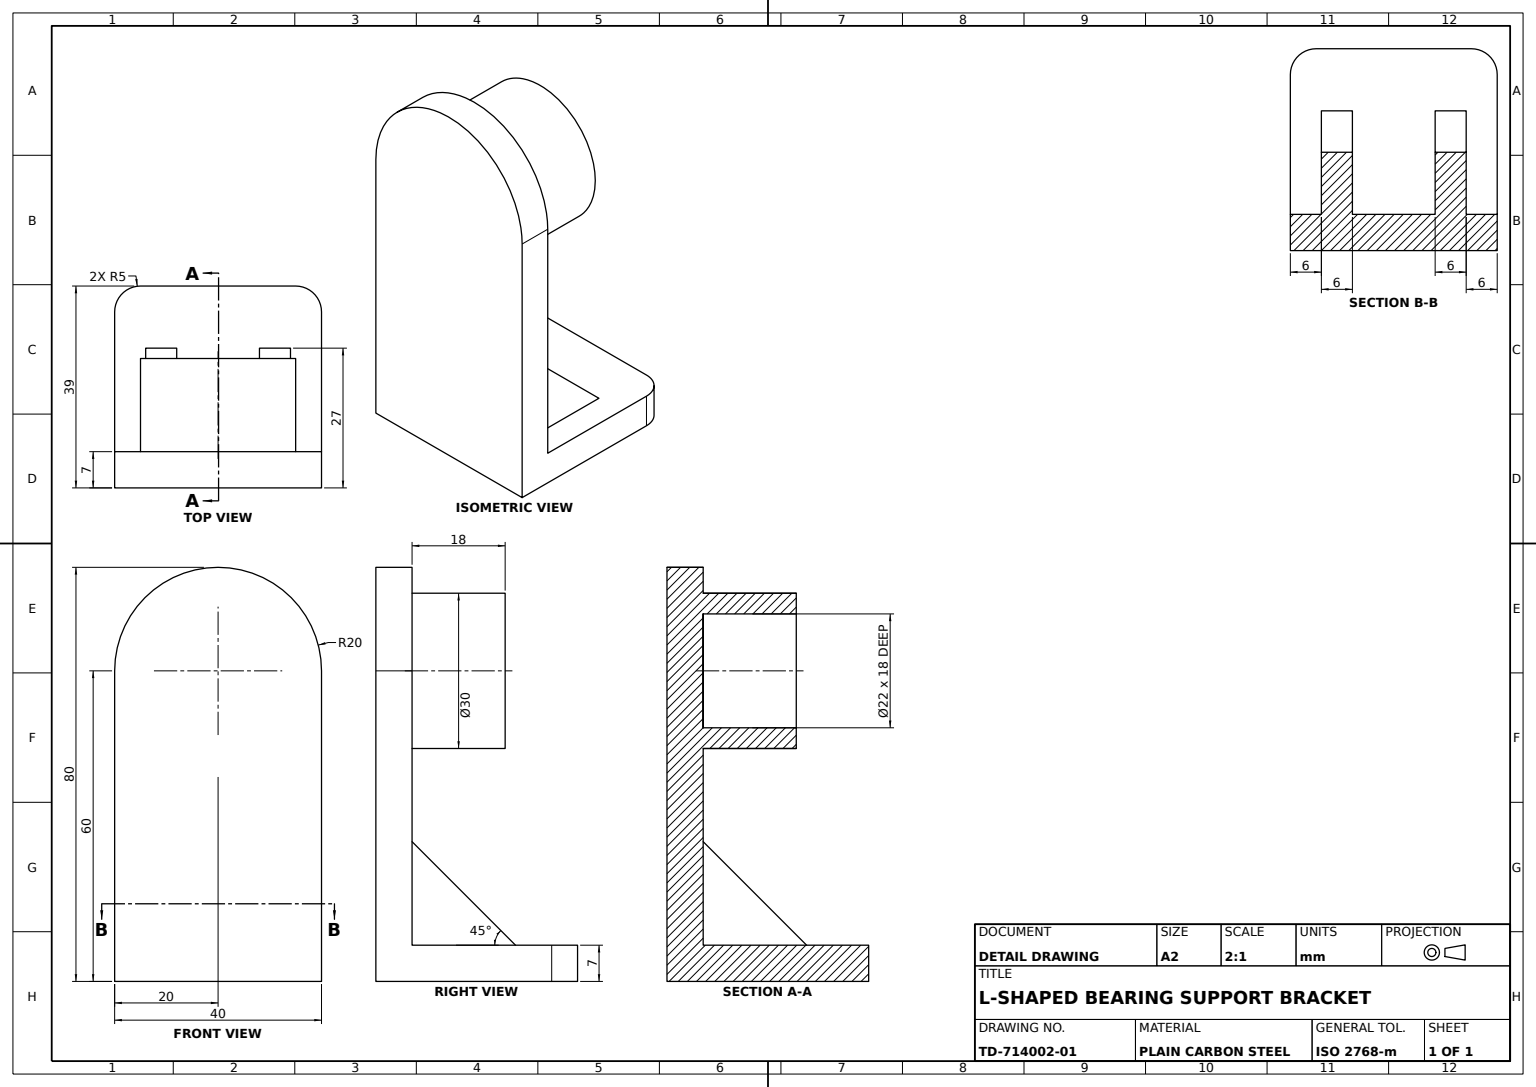
from build123d import *

# Parameters (mm, degrees)
L_BRACKET_BASE_DEPTH      = 40
CORNER_BLOCK_DEPTH        = 7
UPRIGHT_ROUNDED_TOP_DEPTH = 7
HUB_SKETCH_30_R           = 15
HUB_30_DEPTH              = 18
BORE_SKETCH_22_R          = 11
BORE_22_DEPTH             = 18
RIB_1_DEPTH               = 12
RIB_2_DEPTH               = 12
TRIANGULAR_CUT_1_DEPTH    = 6
TRIANGULAR_CUT_2_DEPTH    = 6


with BuildPart() as part:
    # L Profile Sketch → L Bracket Base (new body)
    with BuildSketch(Plane.XY):
        Polygon((0, 0), (34, 0), (34, 60), (27, 60), (27, 7), (0, 7), align=None)
    extrude(amount=L_BRACKET_BASE_DEPTH)

    # Corner Block Sketch → Corner Block (add)
    with BuildSketch(Plane(origin=(0, 7, 0), x_dir=(1, 0, 0), z_dir=(0, 1, 0))):
        with BuildLine():
            Line((-5, -5), (-5, -35))
            ThreePointArc((-5, -35), (-3.535533906, -38.535533906), (0, -40))
            Line((0, -40), (0, 0))
            ThreePointArc((0, 0), (-3.535533906, -1.464466094), (-5, -5))
        make_face()
    extrude(amount=-CORNER_BLOCK_DEPTH)

    # Upright Top Arc Sketch → Upright Rounded Top (add)
    with BuildSketch(Plane.ZY.offset(-27)):
        with BuildLine():
            Line((0, 60), (40, 60))
            ThreePointArc((40, 60), (20, 80), (0, 60))
        make_face()
    extrude(amount=-UPRIGHT_ROUNDED_TOP_DEPTH)

    # Hub Sketch Ø30 → Hub Ø30 (add)
    with BuildSketch(Plane.ZY.offset(-27)):
        with Locations(Location((20, 60, 0), (0, 0, 180))):
            Circle(HUB_SKETCH_30_R)
    extrude(amount=HUB_30_DEPTH)

    # Bore Sketch Ø22 → Bore Ø22 (cut)
    with BuildSketch(Plane.ZY.offset(-9)):
        with Locations((20, 60)):
            Circle(BORE_SKETCH_22_R)
    extrude(amount=-BORE_22_DEPTH, mode=Mode.SUBTRACT)

    # Rib 1 Sketch → Rib 1 (add)
    with BuildSketch(Plane.XY.offset(40)):
        Polygon((27, 7), (27, 27), (7, 7), align=None)
    extrude(amount=-RIB_1_DEPTH)

    # Rib 2 Sketch → Rib 2 (add)
    with BuildSketch(Plane(origin=(0, 0, 0), x_dir=(-1, 0, 0), z_dir=(0, 0, -1))):
        Polygon((-27, 7), (-7, 7), (-27, 27), align=None)
    extrude(amount=-RIB_2_DEPTH)

    # Triangular Cut 1 Sketch → Triangular Cut 1 (cut)
    with BuildSketch(Plane(origin=(0, 0, 0), x_dir=(-1, 0, 0), z_dir=(0, 0, -1))):
        Polygon((-27, 27), (-7, 7), (-27, 7), align=None)
    extrude(amount=-TRIANGULAR_CUT_1_DEPTH, mode=Mode.SUBTRACT)

    # Triangular Cut 2 Sketch → Triangular Cut 2 (cut)
    with BuildSketch(Plane.XY.offset(40)):
        Polygon((27, 27), (7, 7), (27, 7), align=None)
    extrude(amount=-TRIANGULAR_CUT_2_DEPTH, mode=Mode.SUBTRACT)


solid = part.part
